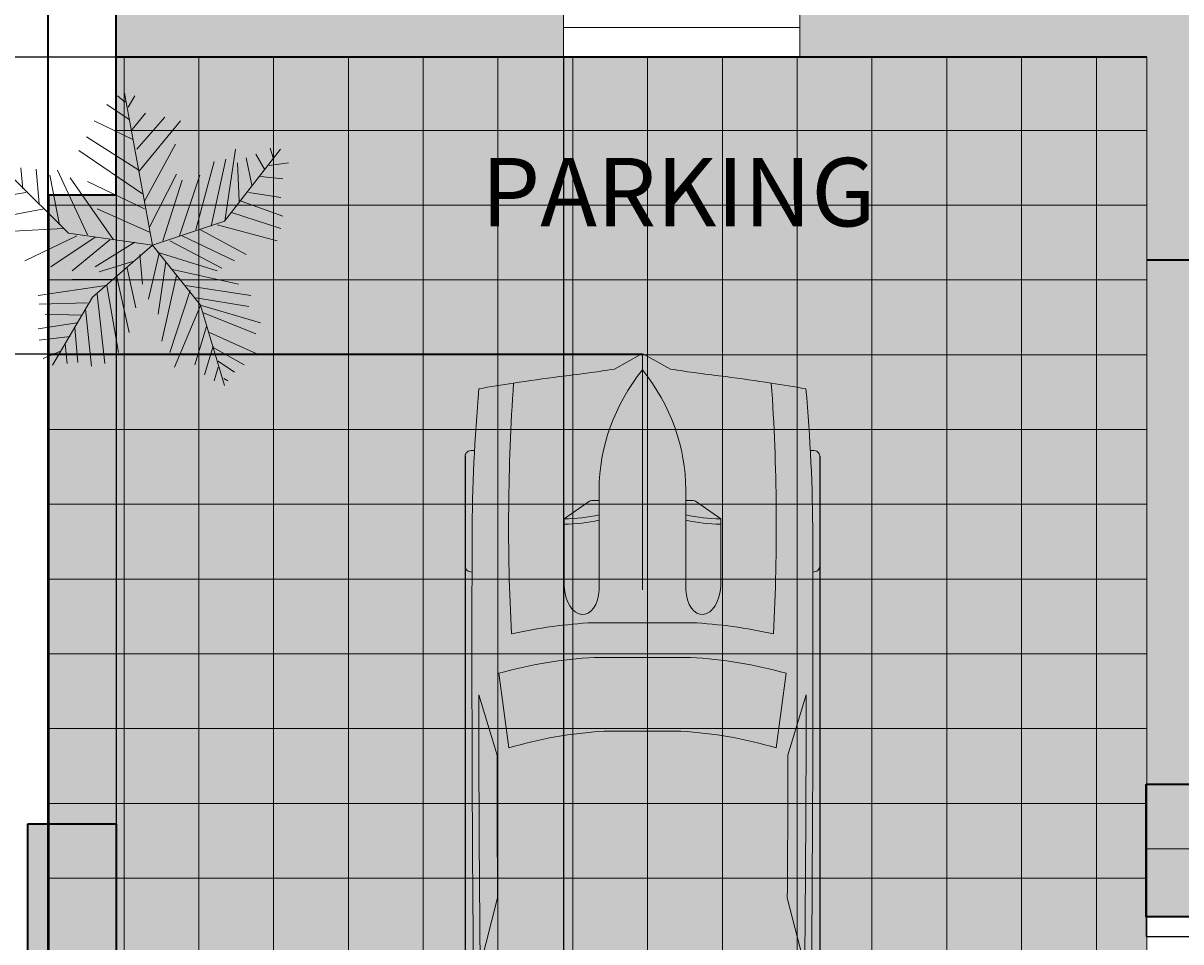
# Model space of a CAD drawing. Units: millimetres. Extents: x -229 to 16545, y -10488 to 4272.
# Tile 1 of 29: x 1930 to 5862, y -7754 to -4633. Entities that reach past the tile are written whole.
import ezdxf

# ---------------------------------------------------------------- set-up
doc = ezdxf.new("R2010")
doc.units = ezdxf.units.MM
for name, color, linetype, lineweight in [('A-ANNO-DIMS', 2, 'Continuous', 18), ('A-AREA-IDEN', 7, 'Continuous', 18), ('A-COLS', 7, 'Continuous', 35), ('A-GLAZ', 4, 'Continuous', 18), ('A-WALL', 7, 'Continuous', 35), ('C-PRKG-VEHI', 8, 'Continuous', 18), ('C-PRKG-VEHI-PATT', 252, 'Continuous', 13), ('L-PLNT-TREE', 80, 'Continuous', 18), ('L-PVMT', 7, 'Continuous', 18), ('L-PVMT-JNTS', 8, 'Continuous', 13)]:
    doc.layers.add(name, color=color, linetype=linetype, lineweight=lineweight)
for name, color, linetype, lineweight, true_color in [('A-FLOR-PATT', 254, 'Continuous', 13, 0xfeeab9), ('A-WALL-PATT', 18, 'Continuous', 13, 0x000000), ('L-PVMT-PATT', 252, 'Continuous', 13, 0x939598)]:
    doc.layers.add(name, color=color, linetype=linetype, lineweight=lineweight, true_color=true_color)
doc.styles.get("Standard").update_dxf_attribs({"font": 'arial.ttf'})
doc.dimstyles.get("Standard").update_dxf_attribs({"dimtxt": 0.18, "dimasz": 0.18, "dimexe": 0.18, "dimexo": 0.0625, "dimgap": 0.09, "dimtad": 0, "dimtih": 1, "dimtoh": 1, "dimdec": 4, "dimzin": 0, "dimdsep": 46, "dimtxsty": 'Standard', "dimcen": 0.09, "dimadec": 0, "dimazin": 0, "dimtfac": 1, "dimtdec": 4, "dimtofl": 0, "dimtmove": 0, "dimatfit": 3, "dimfxl": 1, "dimtolj": 1, "dimtzin": 0, "dimarcsym": 0})

# ---------------------------------------------------------------- blocks, each defined once
blk = doc.blocks.new('*U18')
for p, q in [((0, 0), (-10.5, 57)), ((-8.736999999999625, 47.13799999999969), (-17.06899999999996, 52.71100000000001)), ((-10.18600000000015, 53.63999999999987), (-13.08399999999983, 55.96199999999976)), ((-9.098999999999705, 51.7819999999997), (-6.563000000000101, 55.96199999999976)), ((-7.65000000000009, 43.42299999999977), (-2.577999999999974, 49.45999999999981)), ((-5.838999999999941, 35.99199999999973), (4.666999999999916, 48.06699999999977)), ((-7.28800000000001, 39.70699999999965), (-21.77800000000025, 46.67299999999977)), ((-5.114000000000032, 27.63199999999983), (10.46300000000019, 46.67299999999977)), ((-5.114000000000032, 28.09699999999975), (-24.67599999999993, 40.63599999999996)), ((-3.665000000000418, 19.27299999999968), (-27.57400000000007, 35.52699999999982)), ((-2.940999999999803, 16.48599999999987), (8.652000000000044, 37.84999999999991)), ((27, 9), (48, 36)), ((27.12699999999995, 9.05600000000004), (31.11200000000008, 35.99199999999973)), ((44.15300000000025, 36.45599999999991), (45.23900000000003, 32.74099999999999)), ((16.25900000000001, 5.804999999999836), (23.14199999999983, 31.34799999999973)), ((22.05499999999984, 7.197999999999865), (27.48900000000003, 32.27699999999982)), ((31.83600000000024, 30.88299999999981), (32.56100000000015, 16.48599999999987)), ((35.09600000000001, 32.74099999999999), (37.26999999999998, 22.52399999999989)), ((38.71900000000005, 34.13399999999979), (41.97899999999981, 28.56099999999992)), ((43.79100000000017, 29.95399999999995), (51.03600000000006, 30.88299999999981)), ((-48.58500000000003, 21.13099999999986), (-49.30899999999974, 29.02600000000007)), ((-43.51299999999992, 28.56099999999992), (-42.42699999999968, 15.55799999999976)), ((-38.44199999999955, 26.23899999999981), (-34.81899999999996, 7.662999999999783)), ((-35.54399999999987, 28.09699999999975), (-24.31399999999985, 3.946999999999661)), ((-1.128999999999905, 6.733999999999923), (9.014000000000124, 26.70399999999995)), ((10.10100000000011, 3.482999999999719), (17.70800000000008, 26.23899999999981)), ((-31.5, 4.5), (-52.5, 25.5)), ((-14.5329999999999, 2.089999999999918), (-30.83399999999983, 25.30999999999995)), ((-24.31399999999985, 23.91699999999969), (-2.940999999999803, 13.69999999999982)), ((3.942000000000007, 1.625), (11.1869999999999, 24.38099999999986)), ((40.52999999999975, 25.77499999999986), (48.86200000000008, 24.846)), ((-47.49800000000004, 19.73699999999962), (-55.83000000000038, 18.34399999999982)), ((36.18300000000045, 19.73699999999962), (48.13699999999972, 17.87999999999988)), ((-40.61500000000023, 13.69999999999982), (-55.10500000000002, 10.91299999999978)), ((-20.69099999999981, 13.69999999999982), (-1.128999999999905, 4.875999999999976)), ((33.28499999999986, 16.48599999999987), (48.86200000000008, 10.91299999999978)), ((0, 0), (27, 9)), ((29.66199999999981, 12.30699999999979), (48.13699999999972, 6.268999999999778)), ((-33.37000000000035, 6.268999999999778), (-52.20699999999988, 5.339999999999918)), ((0, 0), (-31.5, 4.5)), ((18.06999999999971, 5.804999999999836), (35.09600000000001, -3.483000000000174)), ((24.22899999999982, 7.662999999999783), (46.6880000000001, 1.625)), ((-28.29899999999998, 3.482999999999719), (-47.86000000000012, -5.805000000000063)), ((-21.41600000000017, 3.017999999999801), (-38.07899999999973, -8.128000000000384)), ((-15.98199999999951, 2.089999999999918), (-30.11000000000013, -9.521000000000186)), ((0, 0), (-22.5, -19.5)), ((-6.563000000000101, 1.161000000000058), (-21.41600000000017, -8.128000000000384)), ((0, 0), (18, -22.5)), ((6.478000000000065, 1.625), (26.03999999999996, -8.592000000000326)), ((11.1869999999999, 3.482999999999719), (30.74900000000025, -5.805000000000063)), ((-4.751999999999952, -3.483000000000174), (-3.665000000000418, -14.62900000000013)), ((2.493000000000392, -3.019000000000005), (-1.490999999999985, -20.20200000000023)), ((1.769000000000232, -2.555000000000063), (24.22899999999982, -9.521000000000186)), ((-6.563000000000101, -5.805000000000063), (-19.96699999999964, -9.985000000000127)), ((-9.460999999999785, -8.592000000000326), (-6.201000000000021, -23.4530000000002)), ((5.028999999999996, -6.270000000000209), (2.131000000000312, -25.77500000000009)), ((-15.2569999999996, -12.77200000000016), (-30.11000000000013, -12.77200000000016)), ((-13.44599999999991, -11.37800000000038), (-8.736999999999625, -32.74100000000021)), ((9.014000000000124, -11.37800000000038), (3.579999999999927, -35.99200000000019)), ((7.564999999999599, -9.056000000000267), (32.19800000000032, -14.62900000000013)), ((-17.43100000000004, -15.09400000000005), (-42.78899999999976, -18.80899999999997)), ((-17.06899999999996, -15.09400000000005), (-12.721, -40.17200000000025)), ((14.08499999999958, -16.95100000000025), (6.478000000000065, -40.17200000000025)), ((12.27399999999988, -15.09400000000005), (36.9069999999997, -18.80899999999997)), ((-24.31399999999985, -21.59600000000023), (-42.42699999999968, -22.06000000000017)), ((-22.5, -19.5), (-37.5, -45)), ((-20.69099999999981, -18.34500000000003), (-17.79300000000012, -44.35200000000032)), ((16.25900000000001, -19.73800000000028), (36.18300000000045, -22.98900000000003)), ((-26.8489999999997, -26.24000000000001), (-40.25300000000015, -25.77500000000009)), ((-25.03800000000001, -23.91800000000035), (-22.86500000000024, -45.28100000000017)), ((18.06999999999971, -22.52400000000012), (8.289000000000215, -45.74500000000012)), ((18, -22.5), (27, -52.5)), ((18.43300000000045, -22.52400000000012), (40.52999999999975, -29.02600000000007)), ((19.1569999999997, -25.31100000000015), (38.71900000000005, -33.20600000000013)), ((-28.29899999999998, -29.02600000000007), (-42.78899999999976, -31.34800000000018)), ((-30.83399999999983, -34.13499999999999), (-42.42699999999968, -35.52800000000025)), ((-29.02300000000014, -30.88400000000002), (-27.93600000000015, -43.88700000000016)), ((20.24400000000014, -30.4190000000001), (15.89699999999993, -44.81600000000026)), ((21.33100000000013, -32.74100000000021), (39.08100000000013, -40.63600000000019)), ((-32.64600000000019, -36.92100000000005), (-31.92099999999982, -44.35200000000032)), ((22.77999999999975, -37.85000000000014), (19.51900000000023, -48.53200000000015)), ((22.77999999999975, -38.31400000000008), (34.37199999999985, -44.81600000000026)), ((-34.45699999999988, -39.70800000000031), (-40.97800000000006, -42.49400000000014)), ((24.59100000000035, -45.74500000000012), (23.14199999999983, -50.85400000000004)), ((24.59100000000035, -43.42300000000022), (30.74900000000025, -47.60300000000029)), ((26.76400000000012, -49.92500000000018), (28.21300000000019, -50.85400000000004))]:
    blk.add_line(p, q)
blk = doc.blocks.new('*U20')
for p, q in [((46.55368679439944, 38.88847654282876), (22.35054758993934, 38.88847654282876)), ((136.6978032355602, 38.88847654282876), (160.90094244002, 38.88847654282867)), ((21.10406751471477, 37.40863046792069), (21.10406751471477, 36.83230215753705)), ((47.80016686962392, 37.39011648242055), (47.80016686962392, 37.40863046792069)), ((87.98532186932616, 31.87120872459877), (74.75900729854769, 35.92175679182955)), ((134.313356548143, 35.6043097713567), (119.2882629232503, 31.77757799177584)), ((135.4513231603356, 37.07354110333037), (135.4513231603356, 37.40863046792069)), ((162.1474225152445, 37.40863046792049), (162.1474225152445, 36.77402019194128)), ((186.4728846989705, -33.49860931502491), (186.4728846989718, 33.49860931502465)), ((70.0302824853563, 31.53613089391356), (86.40615155322342, 29.35124891408057)), ((188.3990091454065, -32.75868627757393), (188.3990091454077, 32.75868627757058)), ((138.4228833961707, 29.35124891408074), (157.2465674415997, 29.35124891408074)), ((186.4728846989718, 29.35124891408083), (167.0083537481071, 29.35124891408083)), ((164.515393597658, 26.39155676426461), (164.5153935976578, -26.39155676426503)), ((32.26591480791686, 11.62530558863241), (36.12873726252356, 17.16961494239206)), ((36.12873726252356, 17.16961494239206), (50.93891189819171, 17.16961494239206)), ((32.12291633764599, 9.505833383620029), (32.12291633764599, 11.15369945057711)), ((58.9167604809788, -10.77488335095668), (58.9167604809788, 10.77488335095617)), ((66.55009204259746, -10.5288681329018), (66.55009204259746, 10.52886813290129)), ((186.4728846989718, -10.5288681329018), (186.4728846989718, 10.52886813290129)), ((29.77279020470884, 9.505833383620029), (51.68362801571248, 9.505833383620029)), ((82.73706193978568, 8.496039918672748), (82.73706193978568, -8.49603991867258)), ((3.266462181856987, 6.128290093440767), (0.1022408397004821, 0.4060708604429806)), ((-4.43e-14, -2.558e-13), (51.68362801571248, -2.558e-13)), ((0.1022408397004821, -0.4060708604432933), (3.266462181856987, -6.128290093441194)), ((29.77279020470884, -9.50583338362054), (51.68362801571248, -9.50583338362054)), ((32.12291633764599, -9.50583338362054), (32.12291633764599, -11.15369945057762)), ((32.26591480791686, -11.62530558863292), (36.12873726252356, -17.16961494239257)), ((36.12873726252356, -17.16961494239257), (50.93891189819171, -17.16961494239257)), ((86.40615155322318, -29.35124891408145), (70.03028248535594, -31.53613089391442)), ((157.2465674415997, -29.35124891408117), (138.4228833961707, -29.35124891408126)), ((167.008353748107, -29.35124891408126), (186.4728846989707, -29.35124891408108)), ((87.98532186932607, -31.87120872459903), (74.7590072985476, -35.92175679182964)), ((134.3133565481428, -35.60430977135721), (119.2882629232503, -31.77757799177618)), ((21.10406751471477, -37.4086304679212), (21.10406751471477, -36.83230215753756)), ((47.80016686962392, -37.39011648242107), (47.80016686962392, -37.4086304679212)), ((135.4513231603355, -37.07354110333088), (135.4513231603355, -37.4086304679212)), ((162.1474225152445, -37.408630467921), (162.1474225152445, -36.77402019194179)), ((46.55368679439944, -38.88847654282927), (22.35054758993934, -38.88847654282927)), ((136.6978032355602, -38.88847654282927), (160.9009424400199, -38.88847654282918))]:
    blk.add_line(p, q)
for centre, major_axis, ratio, start_param, end_param in [((22.35054758993934, 37.40863046792072), (2.08e-14, -1.479846074908118), 0.842303869543976, 3.141592653589776, 4.712388980384677), ((46.55368679439944, 37.40863046792072), (2.2e-14, 1.479846074908118), 0.8423038695439758, -1.570796326794884, 1.73e-14), ((136.6978032355602, 37.40863046792072), (2.357e-13, -1.479846074908118), 0.842303869543976, 3.141592653589603, 4.712388980384554), ((160.90094244002, 37.40863046792052), (5.59e-14, 1.479846074908118), 0.842303869543976, -1.570796326794865, 4.44e-14), ((266.0300214172791, -27.52442688366631), (1.966072e-10, 313.3077612809058), 0.8423038695435284, 1.367075990158062, 1.391760499156098), ((41.19115208863305, -490.8631038926156), (1.294e-13, 528.2339998381949), 0.8423038695439741, 0.0028100083536837, 0.0755983031096952), ((64.48199294511879, -10555.61767587835), (1.907644e-10, 10593.02630634627), 0.842303869543847, -0.0133969486112073, 0.0027970409639888), ((64.4819929449925, -10555.61767590795), (1.9177683e-09, -10591.54646030096), 0.8423038695482963, 3.133765086725325, 3.140440689641252), ((180.6280394947615, 35.8381667808375), (7.4e-14, 2.219769112362114), 0.8423038695439693, -0.0130174256259048, 1.249894140392862), ((64.48199294754608, -10556.35759891604), (1.349839377e-06, 10595.3130398087), 0.8423038681351469, -0.0133969484821159, -0.0130174254969711), ((183.9799245485226, 33.49860931502124), (3e-16, -2.959692149816168), 0.8423038695439952, 1.570796326796048, 3.128195704978389), ((183.9799245485216, 32.75868627756583), (8.56e-14, -5.246425615115243), 0.8423038695439737, 1.570796326795794, 3.128195704978164), ((135.2911776514449, 5.387441675478555), (2.2715e-12, 81.77258453065997), 0.8423038695439563, 1.245306111696802, 1.507880129813836), ((95.78879860270445, -3666.353346297651), (1.949864e-10, -3698.236159209632), 0.8423038695446962, 3.134048706297306, 3.14409775411291), ((259.1750197310735, -27.52442688366614), (1.506617e-10, -305.3028914627677), 0.8423038695443789, 4.528606069860317, 4.561837674556238), ((37.47375371777758, -593.9621830607928), (6.21e-14, -623.32820996736), 0.8423038695439826, 3.09604606856106, 3.200911180495224), ((134.4003789125686, 5.387441675477674), (4.276e-13, -89.7774543484738), 0.84230386954398, 4.44948196380473, 4.652344057257214), ((149.595361812917, 2.799442537139299), (8.561e-13, -79.57966406425402), 0.842303869543983, 4.372215489277867, 4.640744122441986), ((17.08207736189386, -1.421e-13), (6.87e-14, 147.0179238898305), 0.8423038695439764, 4.511394369635731, 4.913383591133647), ((35.90576140732288, -1.421e-13), (6.87e-14, 147.0179238898305), 0.8423038695439764, 4.511394369635731, 4.913383591133647), ((167.0083537481071, 26.39155676426464), (1.394e-13, 2.959692149816236), 0.842303869543976, 5.55e-14, 1.57079632679492), ((-204.4946649195746, 52.39684969293512), (4.12053e-11, -250.9602162198571), 0.8423038695441164, 1.385369446298923, 1.434372047871027), ((13.03653510440275, 17.00972444508943), (1.2303e-12, 27.41599049210566), 0.8423038695439277, 4.435146050259648, 4.718221029521873), ((14.20086229321332, 17.00972444508943), (1.2303e-12, 27.41599049210566), 0.8423038695439277, 4.435146050259648, 4.718221029521873), ((50.7902773840875, 13.33772416300607), (6.340077547122382, -0.356608581037027), 0.6038335755719145, -1.39555193967809, 1.581314658479915), ((32.74615637525823, 11.15369945057713), (1.313e-13, 0.7399230374541176), 0.8423038695439091, 0.8797135699495516, 1.570796326795045), ((29.77279020470884, -46.66302566589627), (5.12e-14, 56.16885904951626), 0.842303869543976, 7e-16, 0.5903187773915901), ((0.6232400376122422, -1.421e-13), (1e-16, -0.7399230374541245), 0.842303869543842, 4.131459131953847, 5.293318828815531), ((29.77279020470884, 46.66302566589578), (4.004e-13, 56.16885904951626), 0.8423038695439734, 2.55127387619821, 3.141592653589801), ((-204.4946649195746, -52.39684969293552), (4.02945e-11, 250.9602162198562), 0.8423038695441192, -1.43437204787103, -1.385369446298926), ((13.03653510440275, -17.00972444508983), (1.2568e-12, -27.41599049210552), 0.8423038695439318, 1.564964277657711, 1.848039256919935), ((14.20086229321332, -17.00972444508983), (1.2568e-12, -27.41599049210552), 0.8423038695439318, 1.564964277657711, 1.848039256919935), ((149.5953618129329, -2.799442537137565), (4.0897e-12, -79.57966406427697), 0.8423038695439419, -1.499151468852248, -1.230622835688196), ((32.74615637525823, -11.1536994505777), (1.3e-13, -0.7399230374541176), 0.8423038695439093, 4.712388980384541, 5.403471737230034), ((134.4003789125684, -5.387441675478584), (4.2949e-12, -89.77745434847827), 0.8423038695439354, -1.510751403667474, -1.307889310215002), ((135.2911776514465, -5.387441675480715), (3.2038e-12, -81.77258453066244), 0.8423038695439492, -1.50788012981387, -1.245306111696839), ((259.1750197310694, 27.52442688365929), (1.08535e-11, 305.3028914629043), 0.8423038695439974, 1.721347632622872, 1.754579237318777), ((167.008353748107, -26.39155676426503), (1.02e-14, -2.959692149816192), 0.8423038695439885, 4.712388980384686, 6.283185307179581), ((266.0300214172791, 27.52442688366566), (8.75241e-11, 313.3077612806533), 0.8423038695441819, 1.749832154434603, 1.774516663432659), ((37.47375371777847, 593.9621830607904), (1.1693e-12, -623.3282099673584), 0.8423038695439528, -0.0593185269054384, 0.0455465850287298), ((95.78879860271888, 3666.35334629765), (1.637818e-10, -3698.236159209629), 0.8423038695447546, -0.0025051005232382, 0.007543947292366), ((183.9799245485177, -32.7586862775633), (2.428e-13, -5.246425615118353), 0.8423038695439808, 0.0133969486110846, 1.570796326792831), ((183.9799245485216, -33.4986093150211), (9.3e-15, 2.959692149816141), 0.8423038695439732, 3.154989602201626, 4.71238898038339), ((41.19115208863322, 490.8631038926152), (1.37757e-11, -528.2339998381949), 0.8423038695440652, -0.0755983031097181, -0.0028100083537155), ((22.35054758993934, -37.40863046792117), (2.2e-14, 1.479846074908118), 0.8423038695439758, 1.570796326794908, 3.14159265358981), ((64.48199294495228, 10555.61767590795), (6.117947e-10, 10593.02630637587), 0.8423038695458146, 3.138795612625926, 3.154989602201039), ((46.55368679439944, -37.40863046792117), (2.08e-14, -1.479846074908118), 0.842303869543976, -1.69e-14, 1.570796326794884), ((64.48199294503607, 10555.61767590793), (1.6049794e-09, -10591.54646030094), 0.8423038695397146, 0.0011519639481523, 0.0078275668641468), ((136.6978032355602, -37.40863046792109), (1.56e-14, -1.479846074908162), 0.8423038695440105, -1.570796326794875, -1.27e-14), ((160.9009424400199, -37.408630467921), (1.969e-13, 1.479846074908162), 0.8423038695440109, 3.141592653589951, 4.712388980384771), ((180.6280394947581, -35.83816678083949), (2.274e-13, -2.219769112363032), 0.8423038695439803, -1.249894138785958, 0.0130174256254374), ((64.48199294197605, 10556.3575989598), (9.365289701e-07, 10595.31303985772), 0.8423038705260315, 3.154610079306566, 3.154989602290631)]:
    blk.add_ellipse(centre, major_axis=major_axis, ratio=ratio, start_param=start_param, end_param=end_param)
at = {"extrusion": (0, 0, -1)}
blk.add_ellipse((50.7902773840875, -13.33772416300655), major_axis=(6.340077547122382, 0.3566085810370246), ratio=0.6038335755719145, start_param=-1.39555193967809, end_param=1.581314658479915, dxfattribs=at)
blk = doc.blocks.new('WIN-802')
at = {"transparency": 33554687}
for p, q in [((0, 145.0133498127079), (0, 229.9999999999991)), ((802.3384173025405, 145.0133498127079), (802.3384173025405, 229.9999999999991)), ((0, 100.7288393788012), (0, -9.095e-13)), ((802.3384173025405, 100.7288393788012), (802.3384173025405, -9.095e-13))]:
    blk.add_line(p, q, dxfattribs=at)
blk.add_lwpolyline([(0, 145.0133498127079), (802.3384173025405, 145.0133498127079), (802.3384173025405, 100.7288393788012), (0, 100.7288393788012)], close=True, dxfattribs=at)
blk = doc.blocks.new('COL-300x450')
at = {"transparency": 33554615}
h = blk.add_hatch(color=256, dxfattribs=at)
h.dxf.hatch_style = 1
h.paths.add_polyline_path([(300, 450), (0, 450), (0, 0), (300, 0)])
at = {"transparency": 33554687}
blk.add_lwpolyline([(0, 450), (300, 450), (300, 0), (0, 0)], close=True, dxfattribs=at)
blk = doc.blocks.new('*D24')
at = {"layer": 'A-ANNO-DIMS', "color": 0, "lineweight": -2, "transparency": 16777216}
for p, q in [((5743.86420577197, -7668.334551523088), (5743.86420577197, -7735.952051523089)), ((6043.86420577197, -7668.334551523088), (6043.86420577197, -7735.952051523089)), ((5744.04420577197, -7735.772051523088), (5893.266252156689, -7735.772051523088)), ((6043.684205771969, -7735.772051523088), (5894.462159387249, -7735.772051523088))]:
    blk.add_line(p, q, dxfattribs=at)
at = {"layer": 'A-ANNO-DIMS', "color": 0, "transparency": 16777216}
for points in [[(5744.04420577197, -7735.742051523089), (5744.04420577197, -7735.802051523087), (5743.86420577197, -7735.772051523088)], [(6043.684205771969, -7735.742051523089), (6043.684205771969, -7735.802051523087), (6043.86420577197, -7735.772051523088)]]:
    blk.add_solid(points, dxfattribs=at)
at = {"layer": 'Defpoints', "color": 0, "transparency": 16777216}
for p in [(5743.86420577197, -7668.272051523088), (6043.86420577197, -7668.272051523088), (6043.86420577197, -7735.772051523088)]:
    blk.add_point(p, dxfattribs=at)
at = {"layer": 'A-ANNO-DIMS', "color": 0, "transparency": 16777216, "insert": (5893.864205771969, -7735.772051523088), "char_height": 0.18, "attachment_point": 5}
blk.add_mtext('\\A1;300 TYP.', dxfattribs=at)
blk = doc.blocks.new('*D62')
at = {"layer": 'A-ANNO-DIMS', "color": 0, "lineweight": -2, "transparency": 16777216}
for p, q in [((5745.870529000002, -4748.272052000002), (-228.8374730000013, -4748.272052000003)), ((-228.6574730000007, -4748.452052000003), (-228.6574730000002, -6998.090148862215)), ((-228.6574729999998, -9248.092052000005), (-228.6574730000002, -6998.453955137795)), ((5745.870529000002, -9248.272052000004), (-228.8374730000003, -9248.272052000006))]:
    blk.add_line(p, q, dxfattribs=at)
at = {"layer": 'A-ANNO-DIMS', "color": 0, "transparency": 16777216}
for points in [[(-228.6874730000008, -4748.452052000003), (-228.6274730000008, -4748.452052000003), (-228.6574730000007, -4748.272052000003)], [(-228.6874729999997, -9248.092052000005), (-228.6274729999997, -9248.092052000005), (-228.6574729999998, -9248.272052000006)]]:
    blk.add_solid(points, dxfattribs=at)
at = {"layer": 'Defpoints', "color": 0, "transparency": 16777216}
for p in [(5745.933029000002, -4748.272052000002), (-228.6574729999998, -9248.272052000006), (5745.933029000002, -9248.272052000004)]:
    blk.add_point(p, dxfattribs=at)
at = {"layer": 'A-ANNO-DIMS', "color": 0, "transparency": 16777216, "insert": (-228.6574730000022, -6998.272052000003), "char_height": 0.18, "attachment_point": 5}
blk.add_mtext('\\A1;4500', dxfattribs=at)
blk = doc.blocks.new('*D91')
at = {"layer": 'A-ANNO-DIMS', "color": 0, "lineweight": -2, "transparency": 16777216}
for p, q in [((2245.933029, -4748.334552), (2245.933028999999, -10230.221103)), ((3765.491243, -4748.334552), (3765.491243, -10230.221103)), ((2246.113028999999, -10230.041103), (3005.257040502046, -10230.041103)), ((3765.311243, -10230.041103), (3006.167231497953, -10230.041103))]:
    blk.add_line(p, q, dxfattribs=at)
at = {"layer": 'A-ANNO-DIMS', "color": 0, "transparency": 16777216}
for points in [[(2246.113028999999, -10230.011103), (2246.113028999999, -10230.071103), (2245.933028999999, -10230.041103)], [(3765.311243, -10230.011103), (3765.311243, -10230.071103), (3765.491243, -10230.041103)]]:
    blk.add_solid(points, dxfattribs=at)
at = {"layer": 'Defpoints', "color": 0, "transparency": 16777216}
for p in [(2245.933029, -4748.272051999999), (3765.491243, -4748.272051999999), (3765.491243, -10230.041103)]:
    blk.add_point(p, dxfattribs=at)
at = {"layer": 'A-ANNO-DIMS', "color": 0, "transparency": 16777216, "insert": (3005.712136, -10230.041103), "char_height": 0.18, "attachment_point": 5}
blk.add_mtext('\\A1;1519.6', dxfattribs=at)
blk = doc.blocks.new('*D95')
at = {"layer": 'A-ANNO-DIMS', "color": 0, "lineweight": -2, "transparency": 16777216}
for p, q in [((3431.620292, -6103.680351), (3431.620292, -10230.221103)), ((4635.562560999999, -6103.680351), (4635.562560999999, -10230.221103)), ((3431.800292, -10230.041103), (4033.241494712823, -10230.041103)), ((4635.382560999999, -10230.041103), (4033.941358287175, -10230.041103))]:
    blk.add_line(p, q, dxfattribs=at)
at = {"layer": 'A-ANNO-DIMS', "color": 0, "transparency": 16777216}
for points in [[(3431.800292, -10230.011103), (3431.800292, -10230.071103), (3431.620292, -10230.041103)], [(4635.382560999999, -10230.011103), (4635.382560999999, -10230.071103), (4635.562560999999, -10230.041103)]]:
    blk.add_solid(points, dxfattribs=at)
at = {"layer": 'Defpoints', "color": 0, "transparency": 16777216}
for p in [(3431.620292, -6103.617851), (4635.562560999999, -6103.617851), (4635.562560999999, -10230.041103)]:
    blk.add_point(p, dxfattribs=at)
at = {"layer": 'A-ANNO-DIMS', "color": 0, "transparency": 16777216, "insert": (4033.591426499999, -10230.041103), "char_height": 0.18, "attachment_point": 5}
blk.add_mtext('\\A1;1204', dxfattribs=at)
blk = doc.blocks.new('*D96')
at = {"layer": 'A-ANNO-DIMS', "color": 0, "lineweight": -2, "transparency": 16777216}
for p, q in [((4033.528927000001, -5757.644295000002), (-228.8374730000011, -5757.644295000003)), ((-228.6574730000006, -5757.824295000003), (-228.6574730000002, -7225.597539470673)), ((-228.6574729999999, -8693.734713000003), (-228.6574730000002, -7225.961468529336)), ((4027.243185000002, -8693.914713000004), (-228.837473, -8693.914713000004))]:
    blk.add_line(p, q, dxfattribs=at)
at = {"layer": 'A-ANNO-DIMS', "color": 0, "transparency": 16777216}
for points in [[(-228.6874730000005, -5757.824295000003), (-228.6274730000005, -5757.824295000003), (-228.6574730000006, -5757.644295000003)], [(-228.6874729999999, -8693.734713000003), (-228.6274729999999, -8693.734713000003), (-228.6574729999999, -8693.914713000004)]]:
    blk.add_solid(points, dxfattribs=at)
at = {"layer": 'Defpoints', "color": 0, "transparency": 16777216}
for p in [(4033.591427000001, -5757.644295000002), (-228.6574729999999, -8693.914713000004), (4027.305685000001, -8693.914713000004)]:
    blk.add_point(p, dxfattribs=at)
at = {"layer": 'A-ANNO-DIMS', "color": 0, "transparency": 16777216, "insert": (-228.6574730000022, -7225.779504000001), "char_height": 0.18, "attachment_point": 5}
blk.add_mtext('\\A1;2936', dxfattribs=at)

msp = doc.modelspace()

# ---------------------------------------------------------------- hatches: boundary and pattern name
at = {"layer": 'A-FLOR-PATT', "transparency": 33554615}
h = msp.add_hatch(color=256, dxfattribs=at)
h.dxf.hatch_style = 1
h.paths.add_polyline_path([(5975.93302901812, -5438.272051523089), (5745.933029018122, -5438.272051523089), (5745.933029018122, -7267.724381862565), (5745.933029018122, -7438.27205152309), (5975.933029018122, -7438.27205152309)])
at = {"layer": 'A-WALL-PATT'}
h = msp.add_hatch(color=256, dxfattribs=at)
h.dxf.hatch_style = 1
h.paths.add_polyline_path([(7294.424812805701, 2163.982606049634), (7294.424812805701, 2251.727948476911), (4412.721615629584, 2251.727948476911), (4412.721615629584, 2166.74129828962), (4412.721615629584, 2122.456787855714), (4412.721615629584, 2021.727948476911), (7294.424812805701, 2021.727948476911), (7294.424812805701, 2119.698095615728)])
h.paths.add_polyline_path([(11407.50963407642, 2166.74129828962), (11407.50963407642, 2251.727948476911), (8296.763230108241, 2251.727948476911), (8296.763230108241, 2163.982606049634), (8296.763230108241, 2119.698095615728), (8296.763230108241, 2021.727948476911), (11407.50963407642, 2021.727948476911), (11407.50963407642, 2122.456787855714)])
h.paths.add_polyline_path([(9785.93302901812, 2021.727948476911), (9555.93302901812, 2021.727948476911), (9555.93302901812, 38.21538932486829), (9705.933029018117, 38.21538932486874, -0.0200240706712671), (9785.93302901812, 35.01025287503762)])
h.paths.add_polyline_path([(14015.93302901812, 2251.727948476911), (12488.00158673236, 2251.727948476911), (12488.00158673236, 2166.741643605608), (12488.00158673236, 2122.738490998308), (12488.00158673236, 2021.727948476911), (13785.93302901812, 2021.727948476911), (13785.93302901812, -2305.464643034989), (13883.90317615694, -2305.464643034989), (13928.18768659085, -2305.464643034989), (14015.93302901812, -2305.464643034989)])
h.paths.add_polyline_path([(13785.93302901813, -978.2720515230884), (9785.93302901812, -978.2720515230884), (9785.93302901812, -961.7846106751313), (9705.93302901812, -961.7846106751313), (9555.93302901812, -961.7846106751317), (9555.93302901812, -1208.272051523088), (13785.93302901812, -1208.272051523088)])
h.paths.add_polyline_path([(5975.93302901812, 2021.727948476911), (5745.933029018121, 2021.727948476911), (5745.933029018121, 755.4922648295469), (5975.93302901812, 755.4922648295469)])
h.paths.add_polyline_path([(2245.93302901812, 2021.727948476911), (3420.864705801971, 2021.727948476911), (3420.864705801971, 2122.456787855714), (3420.864705801971, 2167.10409397907), (3420.864705801971, 2251.727948476911), (2015.93302901812, 2251.727948476911), (2015.93302901812, -3326.810527872243), (2100.942692627708, -3326.810527872243), (2155.198768368638, -3326.810527872243), (2245.933029018121, -3326.810527872243)])
h.paths.add_polyline_path([(5975.93302901812, -397.512652938949), (5745.933029018121, -397.5126529389495), (5745.933029018121, -978.2720515230884), (2245.93302901812, -978.2720515230884), (2245.93302901812, -1208.272051523088), (5975.93302901812, -1208.272051523088)])
h.paths.add_polyline_path([(12015.16993224619, -5208.272051523088), (7975.933029018121, -5208.272051523088), (7975.933029018121, -5325.772051523088), (7975.933029018121, -5438.272051523089), (7975.933029018121, -5596.884208154203), (8205.93302901812, -5596.884208154204), (8205.93302901812, -5438.272051523086), (12015.16993224619, -5438.272051523086), (12015.16993224619, -5337.543212144286), (12015.16993224619, -5293.25870171038)])
h.paths.add_polyline_path([(5975.933029018122, -4518.272051523087), (4567.829660019902, -4518.272051523087), (4567.829660019902, -4603.258701710379), (4567.829660019902, -4647.543212144286), (4567.829660019902, -4748.272051523089), (5745.933029018122, -4748.272051523088), (5745.933029018122, -5438.272051523089), (5975.93302901812, -5438.272051523089), (6475.933029018121, -5438.272051523089), (6475.933029018121, -5325.772051523088), (6475.933029018121, -5208.272051523088), (5975.933029018122, -5208.272051523089)])
h.paths.add_polyline_path([(3765.491242717362, -4518.272051523088), (2245.93302901812, -4518.27205152309), (2245.93302901812, -4748.272051523088), (3765.491242717362, -4748.272051523088), (3765.491242717362, -4647.543212144286), (3765.491242717362, -4603.258701710379)])
at = {"layer": 'C-PRKG-VEHI-PATT'}
h = msp.add_hatch(color=256, dxfattribs=at)
h.dxf.hatch_style = 1
edge = h.paths.add_edge_path()
edge.add_ellipse((3607.529211185457, -9769.523765348671), major_axis=(4725.912256580008, 3.0749239e-09), ratio=0.8423038695445281, start_angle=77.5553727065174, end_angle=79.7904610028182)
edge.add_ellipse((4844.664368095724, -2592.185106036592), major_axis=(3884.719060684347, 1.125906e-09), ratio=0.8423038695442183, start_angle=257.4450673558462, end_angle=260.74343399278183, ccw=False)
edge.add_line((4128.453814510914, -5808.20724164565), (4039.87716894264, -5759.226924584826))
edge.add_ellipse((4033.591426782733, -5767.29169096579), major_axis=(11.45358085171419, 4.4945e-12), ratio=0.8423038695438549, start_angle=52.06686954012766, end_angle=89.99999999999291)
edge.add_line((4033.59142678273, -5757.644295494259), (4033.59142678273, -5810.864491195777))
edge.add_ellipse((3311.274766540754, -6218.509875466019), major_axis=(-869.4614654596021, 1.80077e-11), ratio=0.8423038695439853, start_angle=180.0000000000011, end_angle=209.4385695979805, ccw=False)
edge.add_line((4180.736232000355, -6218.50987546602), (4180.736232000355, -6254.888469336996))
edge.add_line((4180.736232000355, -6254.888469336996), (4208.936604088284, -6254.888469336996))
edge.add_ellipse((4206.244246044127, -6264.535864808529), major_axis=(-11.45358085171833, 5.0922e-12), ratio=0.8423038695436069, start_angle=225.5197891174528, end_angle=270.00000000002547, ccw=False)
edge.add_line((4213.544436413884, -6257.102002985786), (4299.367139905714, -6316.896261388502))
edge.add_line((4299.367139905714, -6316.896261388502), (4299.367139905714, -6546.149202615045))
edge.add_ellipse((4240.051685953036, -6543.848426266054), major_axis=(5.520094670108304, 98.1407350715287), ratio=0.6038335755718915, start_angle=106.3425919543132, end_angle=270.99798572498946, ccw=False)
edge.add_line((4180.736232000355, -6557.67697757519), (4180.736232000355, -6218.50987546602))
edge.add_ellipse((3311.274766540754, -6218.509875466019), major_axis=(-869.4614654596021, 1.80077e-11), ratio=0.8423038695439853, start_angle=180.0000000000011, end_angle=209.4385695979805)
edge.add_ellipse((4755.908087024709, -6218.50987546602), major_axis=(869.4614654596019, 1.2409e-11), ratio=0.842303869543984, start_angle=150.5614304020198, end_angle=179.9999999999992)
edge.add_line((3886.446621565107, -6218.509875466021), (3886.446621565105, -6557.676977575214))
edge.add_ellipse((3827.131167612427, -6543.848426266054), major_axis=(-5.520094670108304, 98.1407350715287), ratio=0.6038335755718915, start_angle=89.0020142750106, end_angle=253.6574080456868, ccw=False)
edge.add_line((3767.815713659748, -6546.149202615045), (3767.815713659748, -6316.896261388502))
edge.add_line((3767.815713659748, -6316.896261388502), (3855.713030733728, -6255.656581488097))
edge.add_ellipse((3860.938607521334, -6264.535864808529), major_axis=(-11.45358085171114, 2.4167e-12), ratio=0.842303869544136, start_angle=-89.99999999998789, end_angle=-45.51978911742532, ccw=False)
edge.add_line((3860.938607521328, -6254.888469336996), (3886.446621565107, -6254.888469336996))
edge.add_line((3886.446621565107, -6254.888469336996), (3886.446621565107, -6218.509875466018))
edge.add_ellipse((4755.908087024709, -6218.50987546602), major_axis=(869.4614654596019, 1.2409e-11), ratio=0.842303869543984, start_angle=150.5614304020199, end_angle=179.9999999999992, ccw=False)
edge.add_line((4033.59142678273, -5810.86449119578), (4033.59142678273, -5757.644295494258))
edge.add_ellipse((4033.591426782733, -5767.29169096579), major_axis=(11.45358085171419, 4.4945e-12), ratio=0.8423038695438549, start_angle=89.99999999999291, end_angle=127.9331304598159)
edge.add_line((4027.305684622828, -5759.226924584826), (3938.729039054555, -5808.207241645646))
edge.add_ellipse((3222.518485469741, -2592.185106036592), major_axis=(3884.719060685492, 7.18321e-11), ratio=0.8423038695439776, start_angle=-80.74343399279951, end_angle=-77.44506735586378, ccw=False)
edge.add_ellipse((4459.653642379904, -9769.523765348607), major_axis=(4725.912256583255, 9.99789e-11), ratio=0.8423038695439494, start_angle=100.2095389971419, end_angle=102.4446272934428)
edge.add_ellipse((13227.78263612094, -6337.716338528086), major_axis=(9648.760328614822, 3.05852e-11), ratio=0.8423038695439373, start_angle=177.1362853921621, end_angle=182.1985405659548)
edge.add_ellipse((3950.196944261551, -7838.084460829144), major_axis=(1389.703090715241, 7.69205e-11), ratio=0.842303869543924, start_angle=94.082410691147, end_angle=107.71995322274691, ccw=False)
edge.add_line((3866.802461740376, -6669.641686482127), (4200.380391825095, -6669.641686482127))
edge.add_ellipse((4116.985909303905, -7838.084460829148), major_axis=(1389.703090715146, 5.3309e-12), ratio=0.8423038695439844, start_angle=72.28004677724942, end_angle=85.91758930884919, ccw=False)
edge.add_ellipse((-5160.599782555511, -6337.716338528068), major_axis=(9648.76032861485, 3.05852e-11), ratio=0.8423038695439409, start_angle=-2.198540565955437, end_angle=2.863714607837381)
edge = h.paths.add_edge_path()
edge.add_ellipse((-159361.2677283546, -6755.788267626439), major_axis=(-163973.9231279127, 1.03867551e-08), ratio=0.8423038695433289, start_angle=179.6161332212111, end_angle=180.0902290885979)
edge.add_ellipse((-159361.2677283546, -6755.788267626439), major_axis=(-163973.9231279127, 1.03867551e-08), ratio=0.8423038695433289, start_angle=180.0902290885979, end_angle=180.1349865768619)
edge.add_ellipse((-3564.68564119695, -6395.259516187628), major_axis=(-8176.756932164527, 2.256357e-10), ratio=0.8423038695440322, start_angle=180.1356123904399, end_angle=182.1799503136467)
edge.add_ellipse((-3564.68564119695, -6395.259516187628), major_axis=(-8176.756932164527, 2.256357e-10), ratio=0.8423038695440322, start_angle=182.1799503136467, end_angle=183.6504275857005)
edge.add_ellipse((3607.529211185454, -9875.635228402642), major_axis=(4849.823013544719, 2.3877334e-09), ratio=0.8423038695443318, start_angle=76.21947101047385, end_angle=77.87403444768762)
edge.add_ellipse((-5160.599782555511, -6337.716338528068), major_axis=(9648.76032861485, 3.05852e-11), ratio=0.8423038695439409, start_angle=-2.1985405659553976, end_angle=2.8637146078373803, ccw=False)
edge.add_ellipse((4116.985909303905, -7838.084460829148), major_axis=(1389.703090715146, 5.3309e-12), ratio=0.8423038695439844, start_angle=72.28004677724944, end_angle=85.91758930884916)
edge.add_line((4200.380391825095, -6669.641686482127), (3866.802461740375, -6669.641686482127))
edge.add_ellipse((3950.196944261551, -7838.084460829144), major_axis=(1389.703090715241, 7.69205e-11), ratio=0.842303869543924, start_angle=94.08241069114707, end_angle=107.7199532227469)
edge.add_ellipse((13227.78263612094, -6337.716338528086), major_axis=(9648.760328614822, 3.05852e-11), ratio=0.8423038695439373, start_angle=177.1362853921622, end_angle=182.1985405659549, ccw=False)
edge.add_ellipse((4459.653642380003, -9875.635228402642), major_axis=(4849.823013547592, 8.133391e-10), ratio=0.8423038695438513, start_angle=102.1259655522744, end_angle=103.7805289894881)
edge.add_ellipse((11631.86849476242, -6395.259516187635), major_axis=(8176.756932164531, 1.784299e-10), ratio=0.8423038695440094, start_angle=176.3495724142996, end_angle=177.8200496863535)
edge.add_ellipse((11631.86849476242, -6395.259516187635), major_axis=(8176.756932164531, 1.784299e-10), ratio=0.8423038695440094, start_angle=177.8200496863535, end_angle=179.8643876095602)
edge.add_ellipse((167428.4505823782, -6755.788267623933), major_axis=(-163973.9231283709, 3.9422692e-09), ratio=0.8423038695444919, start_angle=-0.1349865768556417, end_angle=-0.0902290885918171)
edge.add_ellipse((167428.4505823782, -6755.788267623933), major_axis=(-163973.9231283709, 3.9422692e-09), ratio=0.8423038695444919, start_angle=-0.0902290885918171, end_angle=0.3838667787936917)
edge.add_ellipse((167428.4505823782, -6755.788267623933), major_axis=(-163973.9231283709, 3.9422692e-09), ratio=0.8423038695444919, start_angle=0.3838667787936917, end_angle=0.5282714718187317)
edge.add_ellipse((167428.4505823782, -6755.788267623933), major_axis=(-163973.9231283709, 3.9422692e-09), ratio=0.8423038695444919, start_angle=0.5282714718187317, end_angle=0.6465540970623085)
edge.add_ellipse((3515.052320972862, -8605.547164094223), major_axis=(45.81432340685111, 4.6009e-12), ratio=0.8423038695439874, start_angle=180.6465540970845, end_angle=269.9999999999056)
edge.add_line((3515.052320972781, -8644.136745980357), (3579.251062286293, -8644.136745980357))
edge.add_line((3579.251062286293, -8644.136745980357), (3579.25106228629, -8338.779260567762))
edge.add_ellipse((3625.065385693143, -8342.837059794769), major_axis=(-45.81432340685263, 1.5796e-12), ratio=0.8423038695439878, start_angle=-89.9999999999979, end_angle=1.9895196601282805e-12, ccw=False)
edge.add_line((3625.065385693143, -8304.247477908637), (4446.934968270596, -8304.247477908639))
edge.add_ellipse((4442.11746787232, -8342.837059794772), major_axis=(-45.81432340685263, 2.8e-15), ratio=0.842303869543988, start_angle=180, end_angle=270, ccw=False)
edge.add_line((4487.931791279172, -8342.837059794772), (4487.931791279172, -8644.136745980375))
edge.add_line((4487.931791279172, -8644.136745980373), (4552.130532592662, -8644.136745980375))
edge.add_ellipse((4552.130532592609, -8605.547164094241), major_axis=(-45.81432340685346, 1.7729e-12), ratio=0.8423038695439725, start_angle=90.000000000083, end_angle=179.3534459029321)
edge.add_ellipse((-159361.2677283546, -6755.788267626439), major_axis=(-163973.9231279127, 1.03867551e-08), ratio=0.8423038695433289, start_angle=179.3534459029417, end_angle=179.3813568036844)
edge.add_ellipse((-159361.2677283546, -6755.788267626439), major_axis=(-163973.9231279127, 1.03867551e-08), ratio=0.8423038695433289, start_angle=179.3813568036844, end_angle=179.4717285281857)
edge.add_ellipse((-159361.2677283546, -6755.788267626439), major_axis=(-163973.9231279127, 1.03867551e-08), ratio=0.8423038695433289, start_angle=179.4717285281857, end_angle=179.6161332212111)
edge = h.paths.add_edge_path(flags=16)
edge.add_ellipse((-52719.43876303247, -7240.399519955929), major_axis=(57246.55770143846, 8.170279e-10), ratio=0.842303869544162, start_angle=-0.3640763488911554, end_angle=0.1208973690318383)
edge.add_line((4526.939312293975, -7119.606211509014), (4589.639454651214, -6914.870508417749))
edge.add_ellipse((-159361.2677288128, -6755.788267624483), major_axis=(163951.0159666675, 3.23007761e-08), ratio=0.842303869549042, start_angle=-0.37776419392122307, end_angle=-0.055594313510596294, ccw=False)
edge.add_line((4584.725558298378, -7836.737404937529), (4525.48996268015, -7604.157642007916))
edge = h.paths.add_edge_path(flags=16)
edge.add_line((4165.105212949923, -7038.366181950441), (3902.077640615548, -7038.366181950441))
edge.add_ellipse((3990.257674735825, -8073.294011525872), major_axis=(1231.84719271423, 3.9463e-11), ratio=0.8423038695439561, start_angle=94.87006959713399, end_angle=112.7919148775847)
edge.add_line((3579.251062286288, -7095.161567973676), (3545.430352373573, -6841.672582103935))
edge.add_ellipse((3950.196944261518, -7851.873510313874), major_axis=(1265.792333751566, 7.14673e-11), ratio=0.8423038695439378, start_angle=94.2774209630507, end_angle=111.8349537967049, ccw=False)
edge.add_line((3870.610635088292, -6787.801246035458), (4196.572218477172, -6787.801246035458))
edge.add_ellipse((4116.985909303919, -7851.87351031385), major_axis=(1265.792333751468, 7.9473e-12), ratio=0.8423038695439835, start_angle=68.16504620328988, end_angle=85.72257903694413, ccw=False)
edge.add_line((4521.752501191884, -6841.672582103939), (4487.931791279168, -7095.16156797368))
edge.add_ellipse((4076.925178829671, -8073.294011525625), major_axis=(1231.847192713881, 3.61807e-11), ratio=0.8423038695439931, start_angle=67.20808512240832, end_angle=85.12993040286263)
edge = h.paths.add_edge_path(flags=16)
edge.add_ellipse((4033.591426782733, -6022.064977478797), major_axis=(-2275.752467063544, 5.6979e-12), ratio=0.8423038695439709, start_angle=76.4018653097695, end_angle=103.5981346902307)
edge.add_line((4487.931791279172, -7900.350504724528), (4487.931791279172, -8191.730251303665))
edge.add_ellipse((4033.591426782733, -6313.444724057934), major_axis=(2275.752467063524, 1.15e-12), ratio=0.8423038695439785, start_angle=256.4018653097693, end_angle=283.5981346902305, ccw=False)
edge.add_line((3579.25106228629, -8191.730251303662), (3579.25106228629, -7900.350504724527))
edge = h.paths.add_edge_path(flags=16)
edge.add_line((3541.69289088531, -7604.157642007925), (3482.457295267053, -7836.737404937647))
edge.add_ellipse((167428.450582378, -6755.788267625229), major_axis=(163951.0159666672, 1.7265743e-08), ratio=0.842303869542198, start_angle=180.055594313493, end_angle=180.3777641939035, ccw=False)
edge.add_line((3477.543398914246, -6914.870508417725), (3540.243541271509, -7119.606211509064))
edge.add_ellipse((60786.62161659793, -7240.399519956177), major_axis=(-57246.55770143843, 1.560408e-10), ratio=0.8423038695499789, start_angle=-0.1208973690328125, end_angle=0.364076348890219)
h = msp.add_hatch(color=256, dxfattribs=at)
h.dxf.hatch_style = 1
edge = h.paths.add_edge_path()
edge.add_ellipse((4116.985909303919, -7851.87351031385), major_axis=(1265.792333751468, 7.9473e-12), ratio=0.8423038695439835, start_angle=68.1650462032899, end_angle=85.72257903694413)
edge.add_line((4196.572218477172, -6787.801246035458), (3870.610635088292, -6787.801246035458))
edge.add_ellipse((3950.196944261518, -7851.873510313874), major_axis=(1265.792333751566, 7.14673e-11), ratio=0.8423038695439378, start_angle=94.27742096305064, end_angle=111.8349537967049)
edge.add_line((3545.430352373573, -6841.672582103933), (3579.251062286288, -7095.161567973675))
edge.add_ellipse((3990.257674735825, -8073.294011525872), major_axis=(1231.84719271423, 3.9463e-11), ratio=0.8423038695439561, start_angle=94.87006959713398, end_angle=112.79191487758479, ccw=False)
edge.add_line((3902.077640615549, -7038.366181950441), (4165.105212949924, -7038.366181950441))
edge.add_ellipse((4076.925178829671, -8073.294011525625), major_axis=(1231.847192713881, 3.61807e-11), ratio=0.8423038695439931, start_angle=67.2080851224083, end_angle=85.12993040286261, ccw=False)
edge.add_line((4487.931791279168, -7095.16156797368), (4521.752501191884, -6841.672582103939))
edge = h.paths.add_edge_path()
edge.add_ellipse((4033.591426782733, -6022.064977478797), major_axis=(-2275.752467063544, 5.6979e-12), ratio=0.8423038695439709, start_angle=76.4018653097695, end_angle=103.59813469023078, ccw=False)
edge.add_line((3579.25106228629, -7900.350504724527), (3579.25106228629, -8191.730251303662))
edge.add_ellipse((4033.591426782733, -6313.444724057934), major_axis=(2275.752467063524, 1.15e-12), ratio=0.8423038695439785, start_angle=256.4018653097692, end_angle=283.5981346902305)
edge.add_line((4487.931791279172, -8191.730251303665), (4487.931791279172, -7900.35050472453))
edge = h.paths.add_edge_path()
edge.add_ellipse((4442.11746787232, -8342.837059794772), major_axis=(-45.81432340685263, 2.8e-15), ratio=0.842303869543988, start_angle=180, end_angle=270)
edge.add_line((4442.117467872324, -8304.24747790864), (3625.065385693137, -8304.247477908639))
edge.add_ellipse((3625.065385693143, -8342.837059794769), major_axis=(-45.81432340685263, 1.5796e-12), ratio=0.8423038695439878, start_angle=-89.99999999999801, end_angle=1.9717e-12)
edge.add_line((3579.25106228629, -8342.837059794769), (3579.251062286293, -8644.136745980357))
edge.add_line((3579.251062286293, -8644.136745980357), (4487.931791279172, -8644.136745980371))
edge.add_line((4487.931791279172, -8644.136745980373), (4487.931791279172, -8342.837059794772))
at = {"layer": 'L-PVMT-JNTS', "transparency": 33554523}
h = msp.add_hatch(dxfattribs=at)
h.set_pattern_fill('NET', color=256, scale=80)
h.set_pattern_definition([(0, (-8141.222001159148, -13125.50409224634), (0, 254), []), (90, (-8141.222001159148, -13125.50409224634), (-254, 1.56e-14), [])])
h.paths.add_polyline_path([(5745.933029018122, -5438.272051523089), (5745.933029018122, -4748.272051523088), (2245.933029018121, -4748.272051523088), (2245.933029018121, -5217.29063777321), (2015.933029018121, -5217.29063777321), (2015.93302901812, -9248.272051523089), (5745.933029018122, -9248.272051523089)])
at = {"layer": 'L-PVMT-PATT', "transparency": 33554493}
h = msp.add_hatch(color=256, dxfattribs=at)
h.dxf.hatch_style = 1
h.paths.add_polyline_path([(5745.933029018122, -5438.272051523089), (5745.933029018122, -4748.272051523088), (2245.933029018121, -4748.272051523088), (2245.933029018121, -5217.29063777321), (2015.933029018121, -5217.29063777321), (2015.93302901812, -9248.272051523089), (5745.933029018122, -9248.272051523089)])

# ---------------------------------------------------------------- linework, layer by layer
at = {"layer": 'A-WALL'}
for p, q in [((2015.933029018121, -9248.272051523089), (2015.933029018121, 2251.727948476911)), ((2245.933029018121, -5217.29063777321), (2245.933029018121, 2021.727948476911)), ((5745.933029018122, -4748.272051523088), (2245.933029018121, -4748.272051523088)), ((2245.933029018121, -5217.29063777321), (2015.933029018121, -5217.29063777321)), ((5975.93302901812, -5438.272051523089), (5745.933029018121, -5438.272051523089))]:
    msp.add_line(p, q, dxfattribs=at)
at = {"layer": 'L-PVMT'}
for p, q in [((5745.933029018122, -7267.724381862565), (5745.933029018122, -4748.272051523088)), ((5745.933029018122, -9248.272051523089), (5745.933029018122, -5438.272051523089)), ((5745.933029018122, -7438.27205152309), (8205.93302901812, -7438.27205152309))]:
    msp.add_line(p, q, dxfattribs=at)

# ---------------------------------------------------------------- block references
at = {"layer": 'A-COLS'}
for p in [(5743.86420577197, -7668.272051523088), (1945.93302901812, -7803.015189216731)]:
    msp.add_blockref('COL-300x450', p, dxfattribs=at)
at = {"layer": 'A-GLAZ'}
msp.add_blockref('WIN-802', (3765.491242717362, -4748.272051523087), dxfattribs=at)
at = {"layer": 'C-PRKG-VEHI', "xscale": 15.47942187490615, "yscale": 15.47942187490615, "zscale": 15.47942187490615, "rotation": 270}
msp.add_blockref('*U20', (4033.591426782735, -5757.644295494259), dxfattribs=at)
at = {"layer": 'L-PLNT-TREE', "xscale": 9.061891725250485, "yscale": 9.061891725250485, "zscale": 9.061891725250485}
msp.add_blockref('*U18', (2369.423958503968, -5387.731228287581), dxfattribs=at)

# ---------------------------------------------------------------- texts
at = {"layer": 'A-AREA-IDEN'}
msp.add_text('PARKING', height=232.2974542027223, dxfattribs=at).set_placement((3485.772602074023, -5323.383488936786))

# ---------------------------------------------------------------- dimensions: what is measured, and where the dimension line sits
at = {"layer": 'A-ANNO-DIMS'}
for base, p1, p2, picture, middle in [((-228.6574729999998, -9248.272052000006), (5745.933028999999, -4748.272051999999), (5745.933028999999, -9248.272052), '*D62', (-228.6574730000022, -6998.272052000003)), ((-228.6574729999999, -8693.914713000004), (4033.591427, -5757.644295), (4027.305684999999, -8693.914713), '*D96', (-228.6574730000022, -7225.779504000001))]:
    dim = msp.add_linear_dim(base=base, p1=p1, p2=p2, angle=90, dimstyle='Standard', override={"dimdec": 0, "dimlfac": 1, "dimrnd": 0, "dimzin": 0, "dimdsep": 46, "dimlunit": 2}, dxfattribs=at)
    dim.commit()
    dim.dimension.update_dxf_attribs({"geometry": picture, "text_midpoint": middle})
for base, p1, p2, override, picture, middle in [((3765.491243, -10230.041103), (2245.933029, -4748.272051999999), (3765.491243, -4748.272051999999), {"dimdec": 1, "dimlfac": 1, "dimrnd": 0, "dimzin": 0, "dimdsep": 46, "dimlunit": 2}, '*D91', (3005.712136, -10230.041103)), ((4635.562560999999, -10230.041103), (3431.620292, -6103.617851), (4635.562560999999, -6103.617851), {"dimdec": 0, "dimlfac": 1, "dimrnd": 0, "dimzin": 0, "dimdsep": 46, "dimlunit": 2}, '*D95', (4033.591426499999, -10230.041103))]:
    dim = msp.add_linear_dim(base=base, p1=p1, p2=p2, dimstyle='Standard', override=override, dxfattribs=at)
    dim.commit()
    dim.dimension.update_dxf_attribs({"geometry": picture, "text_midpoint": middle})
dim = msp.add_linear_dim(base=(6043.86420577197, -7735.772051523088), p1=(5743.86420577197, -7668.272051523088), p2=(6043.86420577197, -7668.272051523088), text='<> TYP.', dimstyle='Standard', override={"dimdec": 0, "dimlfac": 1, "dimrnd": 0, "dimzin": 0, "dimdsep": 46, "dimlunit": 2}, dxfattribs=at)
dim.commit()
dim.dimension.update_dxf_attribs({"geometry": '*D24', "text_midpoint": (5893.864205771969, -7735.772051523088)})

doc.saveas('drawing.dxf')
